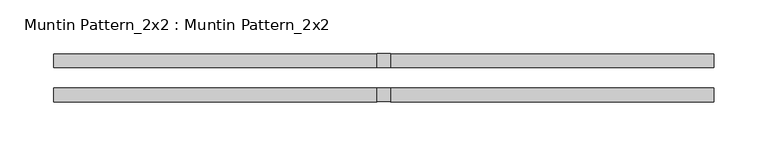
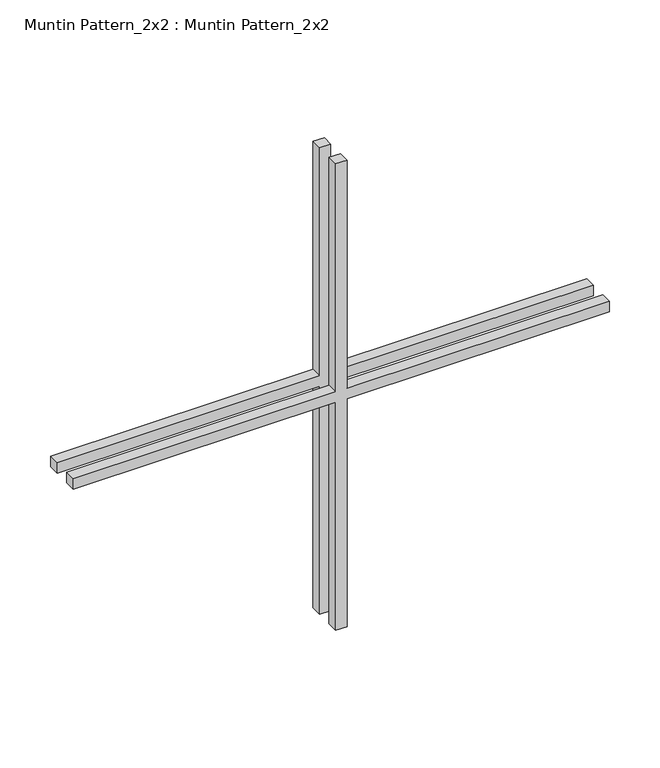
"""IFC4 building model written with IfcOpenShell, lengths in millimetres: proxy geometry, Muntin Pattern_2x2 : Muntin Pattern_2x2."""

from ifc_helpers import new_model, si_unit, frame, origin, place, context, project, spatial, polyline, outline, extrude, source, transform, mapped, element, save


def muntin_pattern_2x2_muntin_pattern_2x2_60a90d43(model_context):
    return source(origin(), model_context, "Body", "SweptSolid", [
        extrude(outline(polyline([(287.3375, -6.35), (287.3375, -305.59375), (274.6375, -305.59375), (274.6375, -6.35), (0.0, -6.35), (0.0, 6.35), (274.6375, 6.35), (274.6375, 305.59375), (287.3375, 305.59375), (287.3375, 6.35), (561.975, 6.35), (561.975, -6.35), (287.3375, -6.35)])), frame((0.0, -22.225, 0.0), z_axis=(0.0, 1.0, 0.0), x_axis=(0.0, 0.0, 1.0)), (0.0, 0.0, 1.0), 12.7),
        extrude(outline(polyline([(287.3375, -6.35), (287.3375, -305.59375), (274.6375, -305.59375), (274.6375, -6.35), (0.0, -6.35), (0.0, 6.35), (274.6375, 6.35), (274.6375, 305.59375), (287.3375, 305.59375), (287.3375, 6.35), (561.975, 6.35), (561.975, -6.35), (287.3375, -6.35)])), frame((0.0, 9.525, 0.0), z_axis=(0.0, 1.0, 0.0), x_axis=(0.0, 0.0, 1.0)), (0.0, 0.0, 1.0), 12.7),
    ])


if __name__ == "__main__":
    model = new_model("IFC4")
    model_context = context("Model", 3, world=origin())
    ifc_project = project(units=[si_unit("LENGTHUNIT", "METRE", prefix="MILLI")], contexts=[model_context])
    site = spatial("IfcSite", under=ifc_project)
    building = spatial("IfcBuilding", under=site)
    placement = place(None, origin())
    muntin_pattern_2x2_muntin_pattern_2x2_shape = muntin_pattern_2x2_muntin_pattern_2x2_60a90d43(model_context)
    element("IfcBuildingElementProxy", 1, Name="Muntin Pattern_2x2 : Muntin Pattern_2x2", ObjectType="Muntin Pattern_2x2 : Muntin Pattern_2x2", at=placement, inside=building, context=model_context, shape_type="MappedRepresentation", body=[
        mapped(muntin_pattern_2x2_muntin_pattern_2x2_shape, transform((0.0, 0.0, 0.0), x_axis=(1.0, 0.0, 0.0), y_axis=(0.0, 1.0, 0.0), z_axis=(0.0, 0.0, 1.0))),
    ])
    save(model, "model.ifc")

# Revit data of these elements
# Type "Muntin Pattern_2x2 : Muntin Pattern_2x2"
#   Width [instance default] = 4' - 0"
#   Thickness = 0' - 0 1/2"
#   Height [instance default] = 4' - 0"
#   Distance = 0' - 0 3/4"
#   Interior Material [instance default] = none
#   Exterior Material [instance default] = none
#   Default Elevation = 0
# Element 1 (IfcBuildingElementProxy, "Muntin Pattern_2x2 : Muntin Pattern_2x2")
#   Width = 2' - 0 1/16"
#   Height = 1' - 10 1/8"
#   Interior Material = Wood - Stained
#   Exterior Material = Clad - White
#   Materials on its faces: "Clad - White", "Wood - Stained"
# Materials
#   "Clad - White": class "Wood", colour RGB 242 242 238, transparency 0, Cost = 0
#   "Wood - Stained": class "Wood", colour RGB 224 178 126, transparency 0, Cost = 0
